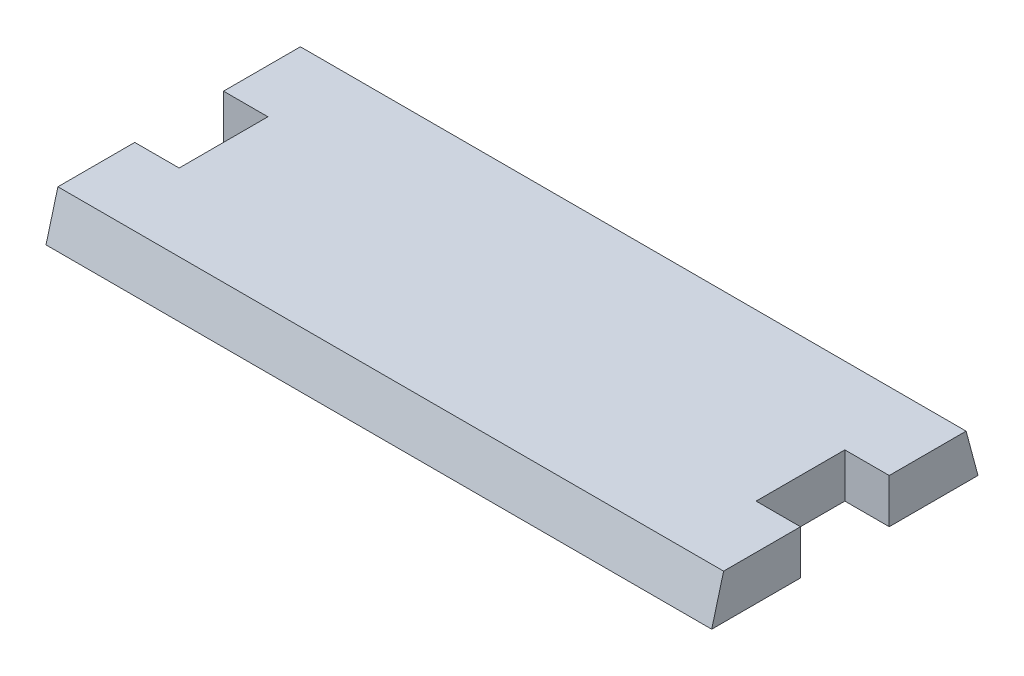
from build123d import *

# Parameters (mm, degrees)
TOP_PLATE_150X60X10_DEPTH = 5
FACE_DRAFT_15_A_ANGLE     = -15
FACE_DRAFT_15_B_ANGLE     = -15


with BuildPart() as part:
    # Top Plate Profile → Top Plate 150x60x10 (new, symmetric)
    with BuildSketch(Plane(origin=(0, 0, 0), x_dir=(1, 0, 0), z_dir=(0, 1, 0))):
        Polygon((0, 0), (150, 0), (150, 20), (140, 20), (140, 40), (150, 40), (150, 60), (0, 60), (0, 40), (10, 40), (10, 20), (0, 20), align=None)
    extrude(amount=TOP_PLATE_150X60X10_DEPTH, both=True)

    # Face Draft 15° A
    face_draft_15_a_faces = [part.faces().sort_by_distance(p)[0] for p in [
        (75, 0, 0),
    ]]
    draft(face_draft_15_a_faces, Plane(origin=(0, -5, 0), x_dir=(0, 0, -1), z_dir=(0, -1, 0)), FACE_DRAFT_15_A_ANGLE)

    # Face Draft 15° B
    face_draft_15_b_faces = [part.faces().sort_by_distance(p)[0] for p in [
        (75, 0, -60),
    ]]
    draft(face_draft_15_b_faces, Plane(origin=(0, -5, 0), x_dir=(0, 0, -1), z_dir=(0, -1, 0)), FACE_DRAFT_15_B_ANGLE)


solid = part.part
